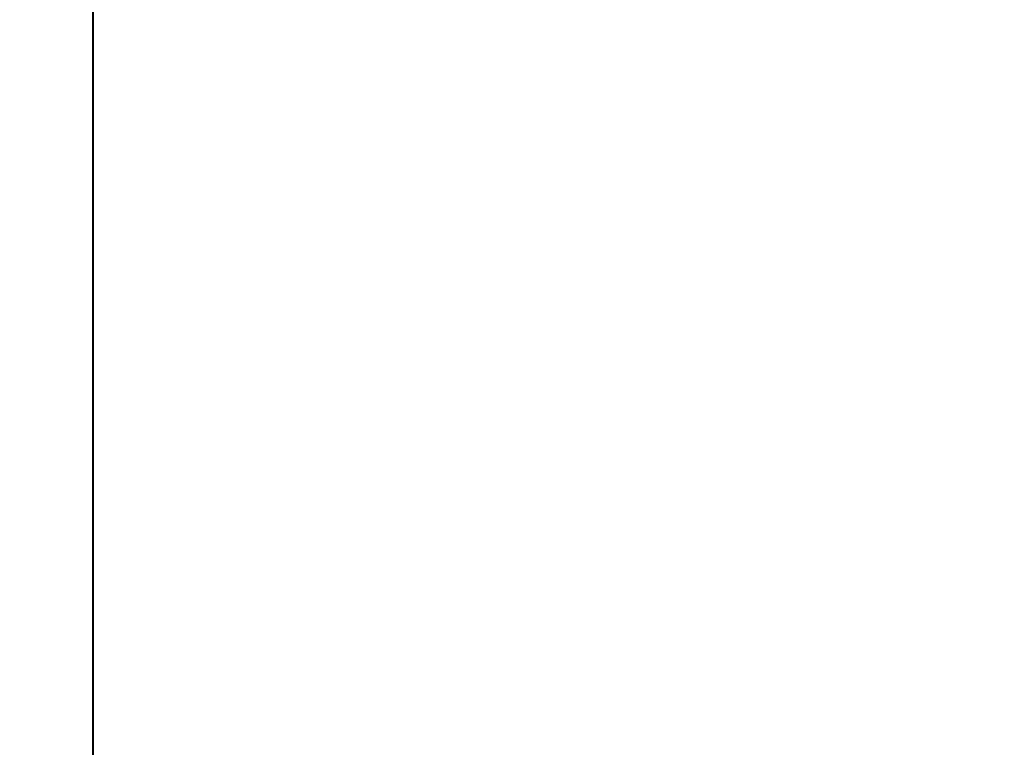
# Model space of a CAD drawing. Units: inches. Extents: x 459864 to 460310, y 324185 to 324787.
# Tile 91 of 112: x 460247.1043 to 460247.2473, y 324283.5352 to 324283.6409. Entities that reach past the tile are written whole.
import ezdxf

# ---------------------------------------------------------------- set-up
doc = ezdxf.new("R2010")
doc.units = ezdxf.units.IN
doc.layers.add('A-ANNO-DIMS', color=2, linetype='Continuous', lineweight=18)
doc.layers.add('A-WALL', color=7, linetype='Continuous', lineweight=40)
doc.styles.get("Standard").update_dxf_attribs({"font": 'arial.ttf'})
doc.dimstyles.new('ISO-25', dxfattribs={"dimtxt": 6, "dimasz": 2.5, "dimexe": 1.25, "dimexo": 0.625, "dimtad": 1, "dimdec": 1, "dimlunit": 3, "dimtxsty": 'Standard', "dimcen": 2.5, "dimadec": 0, "dimazin": 0, "dimtfac": 1, "dimtdec": 1, "dimtmove": 0, "dimatfit": 3, "dimfxl": 1, "dimarcsym": 0})

# ---------------------------------------------------------------- blocks, each defined once
blk = doc.blocks.new('*D21')
at = {"layer": 'A-ANNO-DIMS', "color": 0, "lineweight": -2, "transparency": 16777216}
for p, q in [((460247.73993, 324715.48323), (460309.58037, 324715.48323)), ((460308.33037, 324712.98323), (460308.33037, 324285.98323)), ((460247.73993, 324283.48323), (460309.58037, 324283.48323))]:
    blk.add_line(p, q, dxfattribs=at)
at = {"layer": 'A-ANNO-DIMS', "color": 0, "transparency": 16777216}
for points in [[(460307.9137, 324712.98323), (460308.74704, 324712.98323), (460308.33037, 324715.48323)], [(460307.9137, 324285.98323), (460308.74704, 324285.98323), (460308.33037, 324283.48323)]]:
    blk.add_solid(points, dxfattribs=at)
at = {"layer": 'Defpoints', "color": 0, "transparency": 16777216}
for p in [(460247.11493, 324715.48323), (460247.11493, 324283.48323), (460308.33037, 324283.48323)]:
    blk.add_point(p, dxfattribs=at)
at = {"layer": 'A-ANNO-DIMS', "color": 0, "transparency": 16777216, "insert": (460304.63988, 324499.48323), "char_height": 6, "attachment_point": 5, "rotation": 90}
blk.add_mtext("36'", dxfattribs=at)
blk = doc.blocks.new('*D62')
at = {"layer": 'A-ANNO-DIMS', "color": 0, "lineweight": -2, "transparency": 16777216}
for p, q in [((460247.73993, 324332.73872), (460278.76493, 324332.73872)), ((460277.51493, 324330.23872), (460277.51493, 324285.98323)), ((460247.73993, 324283.48323), (460278.76493, 324283.48323))]:
    blk.add_line(p, q, dxfattribs=at)
at = {"layer": 'A-ANNO-DIMS', "color": 0, "transparency": 16777216}
for points in [[(460277.09826, 324330.23872), (460277.93159, 324330.23872), (460277.51493, 324332.73872)], [(460277.09826, 324285.98323), (460277.93159, 324285.98323), (460277.51493, 324283.48323)]]:
    blk.add_solid(points, dxfattribs=at)
at = {"layer": 'Defpoints', "color": 0, "transparency": 16777216}
for p in [(460247.11493, 324332.73872), (460247.11493, 324283.48323), (460277.51493, 324283.48323)]:
    blk.add_point(p, dxfattribs=at)
at = {"layer": 'A-ANNO-DIMS', "color": 0, "transparency": 16777216, "insert": (460273.78761, 324308.11098), "char_height": 6, "attachment_point": 5, "rotation": 90}
blk.add_mtext('4\'-1 1/2"', dxfattribs=at)
blk = doc.blocks.new('*D67')
at = {"layer": 'A-ANNO-DIMS', "color": 0, "lineweight": -2, "transparency": 16777216}
for p, q in [((460208.11493, 324284.10823), (460208.11493, 324315.13323)), ((460247.11493, 324284.10823), (460247.11493, 324315.13323)), ((460210.61493, 324313.88323), (460244.61493, 324313.88323))]:
    blk.add_line(p, q, dxfattribs=at)
at = {"layer": 'A-ANNO-DIMS', "color": 0, "transparency": 16777216}
for points in [[(460210.61493, 324314.2999), (460210.61493, 324313.46657), (460208.11493, 324313.88323)], [(460244.61493, 324314.2999), (460244.61493, 324313.46657), (460247.11493, 324313.88323)]]:
    blk.add_solid(points, dxfattribs=at)
at = {"layer": 'Defpoints', "color": 0, "transparency": 16777216}
for p in [(460247.11493, 324313.88323), (460208.11493, 324283.48323), (460247.11493, 324283.48323)]:
    blk.add_point(p, dxfattribs=at)
at = {"layer": 'A-ANNO-DIMS', "color": 0, "transparency": 16777216, "insert": (460227.61493, 324317.57372), "char_height": 6, "attachment_point": 5}
blk.add_mtext('3\'-3"', dxfattribs=at)

msp = doc.modelspace()

# ---------------------------------------------------------------- linework, layer by layer
at = {"layer": 'A-WALL'}
msp.add_line((460247.11493, 324470.98323), (460247.11493, 324283.48323), dxfattribs=at)

# ---------------------------------------------------------------- dimensions: what is measured, and where the dimension line sits
at = {"layer": 'A-ANNO-DIMS'}
for base, p1, angle, override, picture, middle in [((460308.33037, 324283.48323), (460247.11493, 324715.48323), 90, {"dimclrd": 0, "dimclre": 0, "dimclrt": 0}, '*D21', (460304.63988, 324499.48323)), ((460277.51493, 324283.48323), (460247.11493, 324332.73872), 270, {"dimdec": 1, "dimlfac": 1, "dimrnd": 0, "dimzin": 1, "dimdsep": 46, "dimlunit": 4, "dimfrac": 2}, '*D62', (460273.78761, 324308.11098))]:
    dim = msp.add_linear_dim(base=base, p1=p1, p2=(460247.11493, 324283.48323), angle=angle, dimstyle='ISO-25', override=override, dxfattribs=at)
    dim.commit()
    dim.dimension.update_dxf_attribs({"geometry": picture, "text_midpoint": middle})
dim = msp.add_linear_dim(base=(460247.11493, 324313.88323), p1=(460208.11493, 324283.48323), p2=(460247.11493, 324283.48323), dimstyle='ISO-25', override={"dimdec": 1, "dimlfac": 1, "dimrnd": 0, "dimzin": 1, "dimdsep": 46, "dimlunit": 4, "dimfrac": 2}, dxfattribs=at)
dim.commit()
dim.dimension.update_dxf_attribs({"geometry": '*D67', "text_midpoint": (460227.61493, 324317.57372)})

doc.saveas('drawing.dxf')
